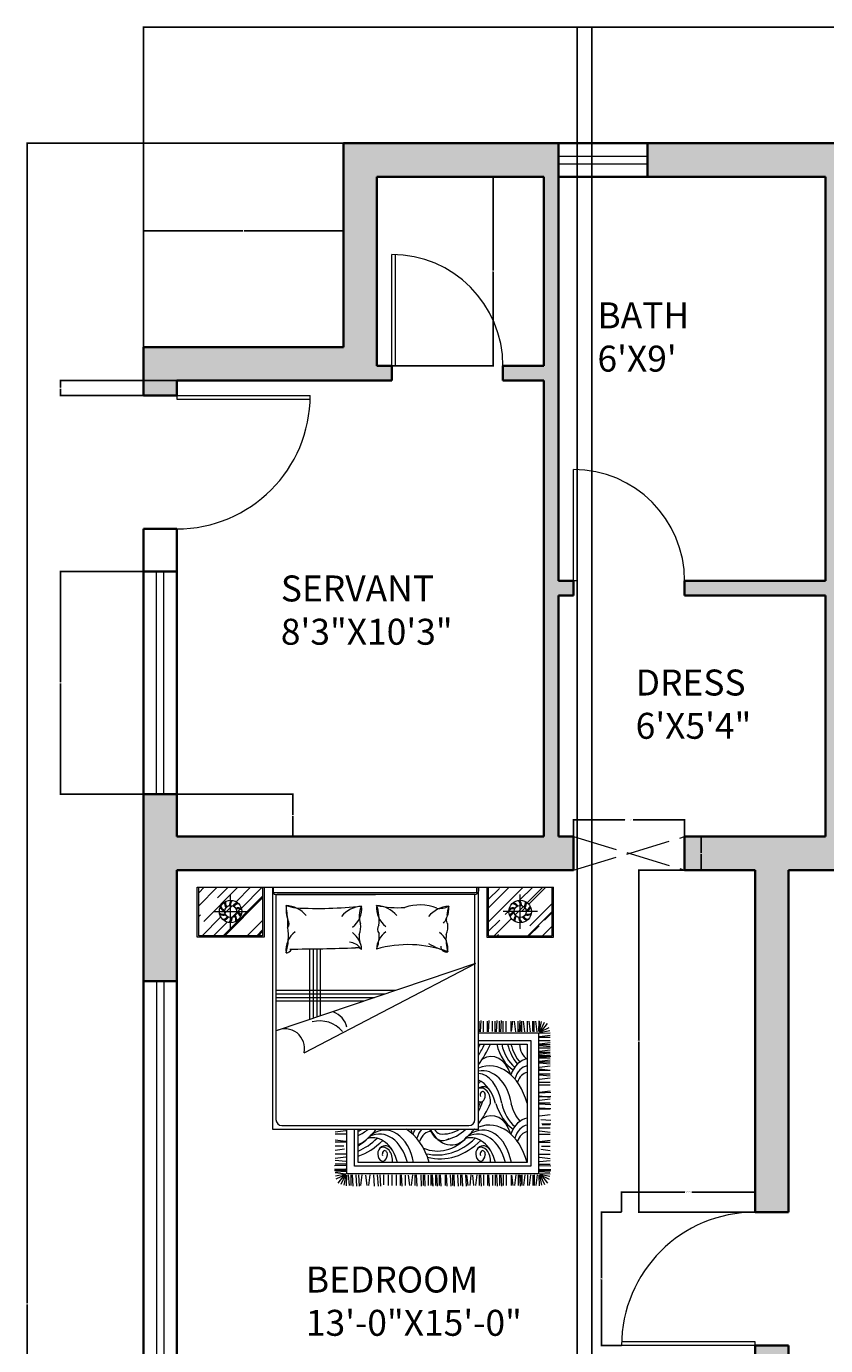
# Model space of a CAD drawing. Units: inches. Extents: x 1919 to 2461, y 2470 to 3159.
# Tile 4 of 6: x 1919 to 2134, y 2803 to 3159. Entities that reach past the tile are written whole.
import ezdxf

# ---------------------------------------------------------------- set-up
doc = ezdxf.new("R2010")
doc.units = ezdxf.units.IN
doc.linetypes.add('ACAD_ISO02W100', pattern=[15, 12, -3])
for name, color, linetype, lineweight in [('A-ANNO-DIMS', 2, 'Continuous', 18), ('A-AREA-IDEN', 7, 'Continuous', 18), ('A-DOOR', 3, 'Continuous', 18), ('A-FURN', 8, 'Continuous', 18), ('A-GLAZ', 4, 'Continuous', 18), ('A-WALL', 7, 'Continuous', 35), ('A-WALL-OVHD', 7, 'ACAD_ISO02W100', 13), ('A-WALL-PATT', 252, 'Continuous', 13)]:
    doc.layers.add(name, color=color, linetype=linetype, lineweight=lineweight)
doc.styles.get("Standard").update_dxf_attribs({"font": 'arial.ttf'})
doc.dimstyles.get("Standard").update_dxf_attribs({"dimtxt": 0.18, "dimasz": 0.18, "dimexe": 0.18, "dimexo": 0.0625, "dimgap": 0.09, "dimtad": 0, "dimtih": 1, "dimtoh": 1, "dimdec": 4, "dimzin": 0, "dimdsep": 46, "dimtxsty": 'Standard', "dimcen": 0.09, "dimadec": 0, "dimazin": 0, "dimtfac": 1, "dimtdec": 4, "dimtofl": 0, "dimtmove": 0, "dimatfit": 3, "dimfxl": 1, "dimtolj": 1, "dimtzin": 0, "dimarcsym": 0})

# ---------------------------------------------------------------- blocks, each defined once
blk = doc.blocks.new('A$C64B41DC1')
for p, q in [((0, 2.508), (2.99, 2.508)), ((0, 2.088), (0, 2.508)), ((0.012, 2.462), (0.058, 2.508)), ((0.012, 2.352), (0.168, 2.508)), ((0.012, 2.1), (0.012, 2.508)), ((0.054, 2.221), (0.341, 2.508)), ((0.169, 2.418), (0.259, 2.508)), ((0.28, 2.16), (0.28, 2.448)), ((0.327, 2.386), (0.448, 2.508)), ((0.37, 2.333), (0.545, 2.508)), ((0.548, 2.508), (0.548, 2.1)), ((0.56, 2.508), (0.56, 2.088)), ((0.63, 2.508), (0.63, 0.478)), ((0.64, 2.461), (0.64, 2.508)), ((0.64, 2.508), (2.344, 2.508)), ((2.344, 2.461), (0.64, 2.461)), ((0.66, 2.446), (1.495, 2.446)), ((0.66, 2.446), (0.66, 0.558)), ((1.495, 2.446), (0.67, 2.446)), ((2.33, 2.446), (1.495, 2.446)), ((2.33, 0.558), (2.33, 2.446)), ((2.344, 2.508), (2.36, 2.508)), ((2.344, 2.508), (2.344, 2.461)), ((2.36, 2.508), (2.36, 2.476)), ((2.36, 0.478), (2.36, 2.508)), ((2.43, 2.508), (2.43, 2.088)), ((2.442, 2.508), (2.442, 2.1)), ((2.442, 2.333), (2.617, 2.508)), ((2.442, 2.214), (2.736, 2.508)), ((2.442, 2.404), (2.535, 2.497)), ((2.705, 2.398), (2.815, 2.508)), ((2.71, 2.16), (2.71, 2.448)), ((2.769, 2.377), (2.9, 2.508)), ((2.782, 2.365), (2.925, 2.508)), ((2.978, 2.1), (2.978, 2.508)), ((2.99, 2.088), (2.99, 2.508)), ((0.216, 2.1), (0.548, 2.432)), ((0.23, 2.1), (0.548, 2.418)), ((0.231, 2.291), (0.294, 2.353)), ((2.667, 2.276), (2.738, 2.346)), ((2.725, 2.308), (2.751, 2.334)), ((2.791, 2.185), (2.978, 2.371)), ((0.012, 2.261), (0.027, 2.276)), ((0.04, 2.1), (0.198, 2.258)), ((0.136, 2.304), (0.425, 2.304)), ((0.137, 2.1), (0.251, 2.214)), ((0.291, 2.254), (0.33, 2.294)), ((0.341, 2.304), (0.36, 2.324)), ((0.419, 2.1), (0.548, 2.229)), ((2.442, 2.135), (2.538, 2.231)), ((2.492, 2.1), (2.637, 2.245)), ((2.854, 2.304), (2.566, 2.304)), ((2.585, 2.278), (2.616, 2.309)), ((2.616, 2.309), (2.631, 2.324)), ((2.775, 2.1), (2.978, 2.304)), ((2.914, 2.231), (2.978, 2.295)), ((0.499, 2.1), (0.548, 2.149)), ((0.513, 2.1), (0.548, 2.135)), ((2.517, 2.1), (2.527, 2.11)), ((2.783, 2.1), (2.868, 2.185)), ((2.896, 2.1), (2.978, 2.182)), ((0.56, 2.088), (0, 2.088)), ((0.548, 2.1), (0.012, 2.1)), ((2.43, 2.088), (2.99, 2.088)), ((2.442, 2.1), (2.978, 2.1)), ((0.942, 1.99), (0.942, 1.397)), ((0.972, 1.991), (0.972, 1.408)), ((1.002, 1.991), (1.002, 1.418)), ((1.032, 1.992), (1.032, 1.428)), ((2.335, 1.868), (0.661, 1.303)), ((0.896, 1.119), (2.335, 1.868)), ((1.664, 1.641), (0.66, 1.641)), ((1.575, 1.611), (0.66, 1.611)), ((2.366, 1.295), (2.366, 1.384)), ((2.377, 1.295), (2.382, 1.389)), ((2.403, 1.295), (2.403, 1.384)), ((2.435, 1.295), (2.435, 1.384)), ((2.445, 1.295), (2.45, 1.389)), ((2.477, 1.296), (2.477, 1.384)), ((2.5, 1.295), (2.5, 1.384)), ((2.51, 1.295), (2.516, 1.389)), ((2.537, 1.295), (2.537, 1.384)), ((2.547, 1.295), (2.552, 1.389)), ((2.568, 1.295), (2.568, 1.384)), ((2.592, 1.295), (2.592, 1.384)), ((2.635, 1.296), (2.635, 1.384)), ((2.636, 1.296), (2.647, 1.384)), ((2.673, 1.295), (2.662, 1.384)), ((2.694, 1.295), (2.694, 1.384)), ((2.704, 1.295), (2.71, 1.389)), ((2.713, 1.296), (2.723, 1.384)), ((2.725, 1.295), (2.725, 1.384)), ((2.749, 1.295), (2.739, 1.384)), ((2.772, 1.295), (2.772, 1.384)), ((2.796, 1.295), (2.785, 1.384)), ((2.815, 1.296), (2.815, 1.384)), ((2.815, 1.296), (2.815, 1.384)), ((2.828, 1.295), (2.828, 1.384)), ((2.828, 1.295), (2.828, 1.384)), ((2.852, 1.295), (2.842, 1.384)), ((2.852, 1.295), (2.842, 1.384)), ((2.865, 1.297), (2.869, 1.386)), ((2.871, 1.296), (2.871, 1.384)), ((2.871, 1.296), (2.888, 1.382)), ((2.871, 1.293), (2.954, 1.332)), ((2.877, 1.296), (2.913, 1.376)), ((2.889, 1.301), (2.939, 1.364)), ((2.36, 1.287), (2.864, 1.287)), ((2.36, 1.223), (2.8, 1.223)), ((2.8, 1.223), (2.8, 0.166)), ((2.864, 1.287), (2.864, 0.102)), ((2.872, 1.288), (2.959, 1.306)), ((2.872, 1.256), (2.96, 1.267)), ((2.872, 1.249), (2.96, 1.249)), ((2.872, 1.221), (2.96, 1.221)), ((2.874, 1.282), (2.96, 1.287)), ((2.36, 1.191), (2.768, 1.191)), ((2.768, 1.191), (2.768, 0.198)), ((2.872, 1.195), (2.96, 1.205)), ((2.872, 1.187), (2.96, 1.187)), ((2.872, 1.181), (2.96, 1.171)), ((2.872, 1.159), (2.96, 1.159)), ((2.872, 1.133), (2.96, 1.143)), ((2.872, 1.125), (2.96, 1.125)), ((2.872, 1.119), (2.96, 1.109)), ((2.872, 1.104), (2.96, 1.093)), ((2.872, 1.097), (2.96, 1.097)), ((2.872, 1.086), (2.966, 1.091)), ((2.872, 1.086), (2.96, 1.075)), ((2.872, 1.076), (2.96, 1.076)), ((2.872, 1.049), (2.96, 1.06)), ((2.872, 1.042), (2.96, 1.042)), ((2.872, 1.035), (2.96, 1.025)), ((2.872, 0.999), (2.96, 1.009)), ((2.872, 0.985), (2.96, 0.974)), ((2.872, 0.973), (2.96, 0.973)), ((2.872, 0.941), (2.96, 0.941)), ((2.872, 0.935), (2.96, 0.924)), ((2.872, 0.898), (2.96, 0.908)), ((2.872, 0.873), (2.96, 0.873)), ((2.872, 0.85), (2.96, 0.85)), ((2.872, 0.789), (2.96, 0.799)), ((2.872, 0.782), (2.966, 0.787)), ((2.872, 0.757), (2.96, 0.747)), ((2.872, 0.75), (2.966, 0.756)), ((2.872, 0.72), (2.96, 0.731)), ((2.872, 0.699), (2.96, 0.699)), ((2.872, 0.689), (2.966, 0.684)), ((2.872, 0.658), (2.966, 0.652)), ((2.872, 0.647), (2.96, 0.647)), ((2.872, 0.59), (2.96, 0.601)), ((2.882, 0.558), (2.966, 0.554)), ((0.63, 0.478), (2.36, 0.478)), ((0.71, 0.508), (2.28, 0.508)), ((1.246, 0.463), (1.158, 0.452)), ((1.254, 0.102), (1.254, 0.478)), ((1.318, 0.166), (1.318, 0.478)), ((1.35, 0.198), (1.35, 0.478)), ((2.872, 0.488), (2.96, 0.488)), ((2.872, 0.463), (2.96, 0.452)), ((2.891, 0.526), (2.966, 0.522)), ((2.893, 0.517), (2.96, 0.517)), ((1.246, 0.437), (1.158, 0.437)), ((1.246, 0.375), (1.158, 0.385)), ((1.246, 0.368), (1.158, 0.368)), ((1.229, 0.336), (1.158, 0.336)), ((2.872, 0.437), (2.96, 0.437)), ((2.872, 0.375), (2.96, 0.385)), ((2.872, 0.368), (2.96, 0.368)), ((2.89, 0.336), (2.96, 0.336)), ((1.235, 0.309), (1.158, 0.3)), ((1.246, 0.268), (1.158, 0.268)), ((1.246, 0.242), (1.158, 0.232)), ((2.872, 0.268), (2.96, 0.268)), ((2.872, 0.242), (2.96, 0.232)), ((2.883, 0.309), (2.96, 0.3)), ((1.246, 0.174), (1.152, 0.169)), ((1.246, 0.143), (1.152, 0.138)), ((1.246, 0.133), (1.152, 0.128)), ((1.246, 0.206), (1.158, 0.216)), ((1.246, 0.185), (1.158, 0.185)), ((1.246, 0.132), (1.158, 0.132)), ((1.246, 0.132), (1.158, 0.132)), ((1.246, 0.123), (1.159, 0.117)), ((2.8, 0.166), (1.318, 0.166)), ((2.768, 0.198), (1.35, 0.198)), ((2.872, 0.206), (2.96, 0.216)), ((2.872, 0.185), (2.96, 0.185)), ((2.872, 0.174), (2.966, 0.169)), ((2.872, 0.143), (2.966, 0.138)), ((2.872, 0.133), (2.966, 0.128)), ((2.872, 0.132), (2.96, 0.132)), ((2.872, 0.123), (2.959, 0.117)), ((1.246, 0.1), (1.158, 0.11)), ((1.246, 0.101), (1.159, 0.083)), ((1.247, 0.096), (1.164, 0.058)), ((1.229, 0.088), (1.179, 0.026)), ((1.242, 0.093), (1.205, 0.013)), ((1.247, 0.093), (1.231, 0.007)), ((1.253, 0.092), (1.249, 0.003)), ((2.864, 0.102), (1.254, 0.102)), ((1.266, 0.094), (1.276, 0.005)), ((1.29, 0.094), (1.29, 0.005)), ((1.3, 0.094), (1.305, 0)), ((1.331, 0.094), (1.337, 0)), ((1.352, 0.094), (1.358, 0)), ((1.38, 0.094), (1.37, 0.005)), ((1.412, 0.093), (1.422, 0.005)), ((1.449, 0.094), (1.438, 0.005)), ((1.48, 0.094), (1.485, 0)), ((1.511, 0.094), (1.517, 0)), ((1.532, 0.094), (1.538, 0)), ((1.564, 0.094), (1.564, 0.01)), ((1.602, 0.094), (1.602, 0.005)), ((1.634, 0.094), (1.634, 0.005)), ((1.67, 0.094), (1.67, 0.005)), ((1.702, 0.094), (1.702, 0.005)), ((1.712, 0.094), (1.717, 0)), ((1.745, 0.093), (1.745, 0.005)), ((1.77, 0.093), (1.78, 0.005)), ((1.806, 0.094), (1.796, 0.005)), ((1.827, 0.094), (1.827, 0.005)), ((1.838, 0.094), (1.843, 0)), ((1.875, 0.094), (1.88, 0)), ((1.896, 0.094), (1.896, 0.005)), ((1.906, 0.094), (1.911, 0)), ((1.938, 0.093), (1.938, 0.005)), ((1.961, 0.094), (1.961, 0.005)), ((1.964, 0.093), (1.974, 0.005)), ((1.971, 0.094), (1.977, 0)), ((1.998, 0.094), (1.998, 0.005)), ((2.008, 0.094), (2.013, 0)), ((2.029, 0.094), (2.029, 0.005)), ((2.039, 0.094), (2.045, 0)), ((2.08, 0.094), (2.08, 0.005)), ((2.09, 0.094), (2.095, 0)), ((2.122, 0.094), (2.127, 0)), ((2.141, 0.094), (2.141, 0.005)), ((2.152, 0.094), (2.157, 0)), ((2.183, 0.094), (2.188, 0)), ((2.209, 0.094), (2.209, 0.005)), ((2.22, 0.094), (2.225, 0)), ((2.251, 0.094), (2.256, 0)), ((2.26, 0.093), (2.271, 0.005)), ((2.297, 0.094), (2.286, 0.005)), ((2.309, 0.093), (2.319, 0.005)), ((2.346, 0.094), (2.335, 0.005)), ((2.366, 0.094), (2.366, 0.005)), ((2.377, 0.094), (2.382, 0)), ((2.403, 0.094), (2.403, 0.005)), ((2.435, 0.094), (2.435, 0.005)), ((2.445, 0.094), (2.45, 0)), ((2.477, 0.093), (2.477, 0.005)), ((2.5, 0.094), (2.5, 0.005)), ((2.51, 0.094), (2.516, 0)), ((2.537, 0.094), (2.537, 0.005)), ((2.547, 0.094), (2.552, 0)), ((2.568, 0.094), (2.568, 0.005)), ((2.592, 0.094), (2.592, 0.005)), ((2.635, 0.093), (2.635, 0.005)), ((2.636, 0.093), (2.647, 0.005)), ((2.673, 0.094), (2.662, 0.005)), ((2.694, 0.094), (2.694, 0.005)), ((2.704, 0.094), (2.71, 0)), ((2.713, 0.093), (2.723, 0.005)), ((2.725, 0.094), (2.725, 0.005)), ((2.749, 0.094), (2.739, 0.005)), ((2.772, 0.094), (2.772, 0.005)), ((2.796, 0.094), (2.785, 0.005)), ((2.815, 0.093), (2.815, 0.005)), ((2.828, 0.094), (2.828, 0.005)), ((2.852, 0.094), (2.842, 0.005)), ((2.865, 0.092), (2.869, 0.003)), ((2.871, 0.096), (2.954, 0.058)), ((2.871, 0.093), (2.888, 0.007)), ((2.872, 0.101), (2.959, 0.083)), ((2.874, 0.107), (2.96, 0.102)), ((2.877, 0.093), (2.913, 0.013)), ((2.889, 0.088), (2.939, 0.026))]:
    blk.add_line(p, q)
at = {"ltscale": 10}
for p, q in [((1.486, 1.581), (0.66, 1.581)), ((1.397, 1.551), (0.66, 1.551))]:
    blk.add_line(p, q, dxfattribs=at)
for centre, radius in [((0.28, 2.304), 0.0942), ((0.28, 2.304), 0.051), ((2.71, 2.304), 0.0942), ((2.71, 2.304), 0.051)]:
    blk.add_circle(centre, radius)
for centre, radius, start, end in [((0.66, 2.476), 0.03, 180, 270), ((2.33, 2.476), 0.03, 270, 0), ((0.246, 2.366), 0.0605, 208.17, 254.4897), ((0.242, 2.361), 0.0462, 196.3002, 256.538), ((0.289, 2.374), 0.0605, 172.17, 218.4897), ((0.283, 2.373), 0.0462, 160.3002, 220.538), ((0.329, 2.356), 0.0605, 136.17, 182.4897), ((0.323, 2.358), 0.0462, 124.3002, 184.538), ((0.35, 2.318), 0.0605, 100.17, 146.4897), ((0.347, 2.323), 0.0462, 88.3002, 148.538), ((0.345, 2.274), 0.0605, 64.17, 110.4897), ((0.345, 2.28), 0.0462, 52.3002, 112.538), ((1.053, 2.33), 0.308, 175.3048, 198.6942), ((-0.87, 2.094), 1.636, 4.8098, 9.1892), ((0.858, 2.628), 0.295, 247.5179, 264.267), ((0.728, 2.111), 0.245, 40.4189, 85.9871), ((1.016, 5.71), 3.38, 266.8134, 276.1602), ((1.396, 2.104), 0.245, 94.0129, 139.5811), ((1.186, 2.329), 0.194, 306.5711, 5.89), ((1.535, 2.265), 0.177, 151.7736, 201.6983), ((1.699, 2.335), 0.194, 174.11, 233.4289), ((1.148, 2.231), 0.378, 353.4947, 19.1867), ((1.687, 3.192), 0.856, 257.7438, 273.6284), ((1.488, 2.111), 0.245, 40.4189, 85.9871), ((1.867, 1.971), 0.388, 68.2026, 108.9817), ((2.127, 2.104), 0.245, 94.0129, 139.5811), ((2.034, 2.486), 0.156, 261.5958, 298.9092), ((1.916, 2.329), 0.194, 333.7371, 5.89), ((2.606, 2.203), 0.517, 163.6046, 172.3273), ((2.645, 2.28), 0.0462, 67.462, 127.6998), ((2.645, 2.274), 0.0605, 69.5103, 115.83), ((2.643, 2.323), 0.0462, 31.462, 91.6998), ((2.64, 2.318), 0.0605, 33.5103, 79.83), ((2.667, 2.358), 0.0462, 355.462, 55.6998), ((2.662, 2.356), 0.0605, 357.5103, 43.83), ((2.707, 2.373), 0.0462, 319.462, 19.6998), ((2.702, 2.374), 0.0605, 321.5103, 7.83), ((2.749, 2.361), 0.0462, 283.462, 343.6998), ((2.745, 2.366), 0.0605, 285.5103, 331.83), ((0.215, 2.328), 0.0462, 232.3002, 292.538), ((0.216, 2.334), 0.0605, 244.17, 290.4897), ((0.214, 2.285), 0.0462, 268.3002, 328.538), ((0.211, 2.29), 0.0605, 280.17, 326.4897), ((0.238, 2.249), 0.0462, 304.3002, 4.538), ((0.232, 2.252), 0.0605, 316.17, 2.4897), ((0.278, 2.235), 0.0462, 340.3002, 40.538), ((0.272, 2.233), 0.0605, 352.17, 38.4897), ((0.319, 2.246), 0.0462, 16.3002, 76.538), ((0.315, 2.242), 0.0605, 28.17, 74.4897), ((0.727, 2.201), 0.0446, 314.4736, 42.1713), ((-1.601, 2.277), 2.362, 357.3905, 358.8876), ((1.916, 2.329), 0.194, 320.9404, 333.7371), ((2.135, 2.231), 0.0459, 165.3506, 223.2684), ((2.675, 2.242), 0.0605, 105.5103, 151.83), ((2.671, 2.246), 0.0462, 103.462, 163.6998), ((2.718, 2.233), 0.0605, 141.5103, 187.83), ((2.712, 2.235), 0.0462, 139.462, 199.6998), ((2.758, 2.252), 0.0605, 177.5103, 223.83), ((2.753, 2.249), 0.0462, 175.462, 235.6998), ((2.78, 2.29), 0.0605, 213.5103, 259.83), ((2.777, 2.285), 0.0462, 211.462, 271.6998), ((2.774, 2.334), 0.0605, 249.5103, 295.83), ((2.775, 2.328), 0.0462, 247.462, 307.6998), ((0.938, 1.978), 0.194, 126.5711, 185.89), ((0.269, 2.094), 0.496, 344.0243, 8.7071), ((1.186, 1.971), 0.194, 4.3181, 53.4289), ((1.541, 2.097), 0.183, 175.2233, 196.23), ((1.204, 2.178), 0.168, 337.017, 7.5368), ((1.706, 1.971), 0.204, 127.1197, 175.09), ((1.567, 2.155), 0.0547, 142.0833, 220.902), ((1.196, 2.098), 0.33, 343.7954, 3.5554), ((1.939, 1.991), 0.165, 351.2621, 55.7572), ((2.462, 2.072), 0.375, 173.8296, 196.4356), ((1.935, 2.178), 0.168, 337.017, 7.5368), ((0.725, 18.844), 16.855, 270.174, 272.0521), ((1.269, 1.925), 0.122, 33.628, 86.4744), ((1.34, 1.94), 0.0603, 49.0991, 101.3702), ((1.768, 1.063), 0.963, 69.6507, 105.9631), ((2.275, 2.579), 0.637, 238.3499, 254.3137), ((2.091, 2.012), 0.0478, 179.7727, 283.8018), ((0.742, 2.015), 0.057, 273.4709, 328.5412), ((0.728, 2.202), 0.245, 274.0129, 278.3417), ((1.075, 1.287), 0.187, 14.1863, 69.1212), ((1.027, 1.133), 0.253, 40.629, 104.3712), ((0.735, 1.155), 0.165, 347.3109, 116.4454), ((0.71, 0.558), 0.05, 180, 270), ((2.28, 0.558), 0.05, 270, 0)]:
    blk.add_arc(centre, radius, start, end)
for centre, major_axis, ratio, start_param, end_param in [((1.994, 1.626), (0, -0.753), 0.68, 0.797284, 0.954936), ((2.064, 1.466), (0, -0.532), 0.68, 7.239912, 7.311536), ((1.905, 1.74), (0, -0.984), 0.68, 0.74745, 0.979724), ((2.467, 0.822), (0, -0.266), 0.68, 2.006169, 3.565187), ((2.746, 1.308), (0, 0.361), 0.68, 1.900046, 2.742661), ((2.787, 1.308), (0, 0.361), 0.68, 1.900046, 2.614747), ((2.837, 1.308), (0, 0.361), 0.68, 1.900046, 2.479658), ((2.861, 1.321), (0, 0.361), 0.68, 1.938265, 2.479658), ((2.806, 1.208), (0, -0.152), 0.68, 4.821745, 5.895886), ((2.451, 0.507), (0, 0.502), 0.68, 5.095327, 6.553458), ((2.786, 0.807), (0, -0.261), 0.68, 3.244645, 4.205018), ((2.778, 0.829), (0, -0.18), 0.68, 3.227058, 4.318474), ((2.396, 0.603), (0, 0.364), 0.68, -1.3172, 0.145284), ((2.351, 0.564), (0.007, 0.382), 0.56205, -1.21172, -0.009991), ((2.296, 0.577), (0, -0.326), 0.68, 1.938944, 2.850232), ((2.782, 0.797), (0, -0.159), 0.68, 3.272942, 4.229533), ((2.04, 1.601), (0, -0.876), 0.68, 6.849801, 6.887077), ((2.4, 0.713), (0, -0.121), 0.68, 2.284368, 3.652258), ((2.383, 0.708), (0, 0.115), 0.68, 4.593909, 6.585576), ((2.396, 0.763), (0, -0.0317), 0.68, 1.462497, 5.046281), ((2.377, 0.765), (0, -0.0593), 0.68, 5.841311, 7.755362), ((1.994, 1.13), (-0.068, 0.744), 0.610498, 3.917146, 4.063997), ((2.064, 0.969), (0, -0.532), 0.68, 7.239912, 7.336618), ((1.905, 1.243), (0, -0.984), 0.68, 0.74745, 0.979724), ((2.746, 0.811), (-0.06, 0.373), 0.695517, 1.775813, 2.548612), ((2.787, 0.811), (0, 0.361), 0.68, 1.900046, 2.614747), ((2.861, 0.824), (0, 0.361), 0.68, 1.938265, 2.479658), ((2.451, 0.01), (0, 0.502), 0.68, 5.095327, 6.553458), ((2.467, 0.325), (0, -0.266), 0.68, 2.006169, 3.565187), ((2.786, 0.31), (0, -0.261), 0.68, 3.244645, 4.205018), ((1.242, 0.969), (0, -0.532), 0.68, 6.586764, 6.677612), ((1.171, 1.13), (-0.116, 0.724), 0.59432, 3.291697, 3.50733), ((1.083, 1.243), (0, -0.984), 0.68, 0.565948, 0.680366), ((1.528, 0.067), (0, -0.37), 0.68, 1.930561, 3.464283), ((1.574, 0.106), (0, 0.364), 0.68, -1.3172, 0.476403), ((1.629, 0.01), (0, 0.502), 0.68, 6.655152, 6.661293), ((1.629, 0.01), (0, 0.502), 0.68, 5.095327, 5.911219), ((1.644, 0.325), (0, -0.266), 0.68, 2.006169, 2.182797), ((1.964, 0.31), (0, -0.261), 0.68, 4.015924, 4.205018), ((1.956, 0.332), (0, -0.18), 0.68, 3.770744, 4.318474), ((1.96, 0.3), (0, -0.159), 0.68, 3.14258, 4.229533), ((2.061, 0.562), (0, -0.18), 0.68, 5.194792, 5.929328), ((2.061, 0.562), (0, -0.18), 0.68, 5.194792, 6.723255), ((2.131, 0.66), (0, -0.315), 0.68, 5.328638, 6.949396), ((2.055, 0.566), (0, -0.13), 0.68, 5.450951, 6.054641), ((2.064, 0.969), (0, -0.532), 0.68, 6.20013, 6.677612), ((1.994, 1.13), (-0.068, 0.744), 0.610498, 3.199135, 3.592282), ((1.905, 1.243), (0, -0.984), 0.68, 0.565948, 0.680366), ((2.351, 0.067), (0, -0.37), 0.68, 1.930561, 3.464283), ((2.396, 0.106), (0, 0.364), 0.68, -1.3172, 0.476403), ((2.451, 0.01), (0, 0.502), 0.68, 6.655152, 6.661293), ((2.778, 0.332), (0, -0.18), 0.68, 3.227058, 4.318474), ((2.782, 0.3), (0, -0.159), 0.68, 3.272942, 4.229533), ((1.193, 0.918), (0, -0.624), 0.68, 0.378672, 0.625379), ((1.309, 0.66), (0, -0.315), 0.68, 6.475719, 6.949396), ((1.191, 1.107), (0, 0.846), 0.68, 3.421828, 3.728616), ((1.218, 1.105), (0, -0.876), 0.68, 6.507006, 6.887077), ((1.474, 0.08), (0, -0.326), 0.68, 1.938944, 3.339184), ((1.578, 0.217), (0, -0.121), 0.68, 2.284368, 3.726131), ((1.561, 0.211), (0, 0.115), 0.68, 4.593909, 6.647252), ((2.016, 0.918), (0, -0.624), 0.68, -0.280078, 0.625379), ((2.013, 1.107), (0, 0.846), 0.68, 2.978727, 3.728616), ((2.04, 1.105), (0, -0.876), 0.68, 6.099302, 6.887077), ((2.296, 0.08), (0, -0.326), 0.68, 1.938944, 3.339184), ((2.4, 0.217), (0, -0.121), 0.68, 2.284368, 3.726131), ((2.383, 0.211), (0, 0.115), 0.68, 4.593909, 6.647252), ((1.555, 0.269), (0, -0.0593), 0.68, 3.732151, 7.755362), ((1.574, 0.266), (0, -0.0317), 0.68, 1.462497, 5.046281), ((2.377, 0.269), (0, -0.0593), 0.68, 3.732151, 7.755362), ((2.396, 0.266), (0, -0.0317), 0.68, 1.462497, 5.046281)]:
    blk.add_ellipse(centre, major_axis=major_axis, ratio=ratio, start_param=start_param, end_param=end_param)
blk = doc.blocks.new('DOOR-SGL-30IN')
for p, q in [((0, 0), (0, 30)), ((1, 0), (1, 29.98)), ((1, 0), (0, 0))]:
    blk.add_line(p, q)
blk.add_arc((0, 0), 30, 0, 90)
blk = doc.blocks.new('DOOR-SGL-36IN')
for p, q in [((0, 0), (-36, 0)), ((0, 1), (-35.99, 1)), ((0, 0), (0, 1))]:
    blk.add_line(p, q)
blk.add_arc((0, 0), 36, 90, 180)
blk = doc.blocks.new('WIN-GLAZ-120IN')
for p, q in [((120, 0), (0, 0)), ((120, -2), (0, -2))]:
    blk.add_line(p, q)
blk = doc.blocks.new('WIN-GLAZ-24IN')
for p, q in [((-2, 24), (-2, 0)), ((0, 24), (0, 0))]:
    blk.add_line(p, q)
blk = doc.blocks.new('OPENING-OVHD-30IN')
for p, q in [((0, 0), (9, 30)), ((9, 0), (0, 30))]:
    blk.add_line(p, q)
blk = doc.blocks.new('*D13')
at = {"layer": 'A-ANNO-DIMS', "color": 0, "lineweight": -2, "transparency": 16777216}
for p, q in [((2079.32, 2839.46), (2079.32, 2844.98)), ((2079.5, 2844.8), (2096.38, 2844.8)), ((2115.14, 2844.8), (2098.25, 2844.8)), ((2115.32, 2839.46), (2115.32, 2844.98))]:
    blk.add_line(p, q, dxfattribs=at)
at = {"layer": 'A-ANNO-DIMS', "color": 0, "transparency": 16777216}
for points in [[(2079.5, 2844.83), (2079.5, 2844.77), (2079.32, 2844.8)], [(2115.14, 2844.83), (2115.14, 2844.77), (2115.32, 2844.8)]]:
    blk.add_solid(points, dxfattribs=at)
at = {"layer": 'Defpoints', "color": 0, "transparency": 16777216}
for p in [(2115.32, 2844.8), (2079.32, 2839.4), (2115.32, 2839.4)]:
    blk.add_point(p, dxfattribs=at)
at = {"layer": 'A-ANNO-DIMS', "color": 0, "transparency": 16777216, "insert": (2097.32, 2844.8), "char_height": 0.18, "attachment_point": 5}
blk.add_mtext('\\A1;DOOR 36 TYP.', dxfattribs=at)
blk = doc.blocks.new('*D14')
at = {"layer": 'A-ANNO-DIMS', "color": 0, "lineweight": -2, "transparency": 16777216}
for p, q in [((2079.25, 2839.4), (2073.74, 2839.4)), ((2073.92, 2839.22), (2073.92, 2821.58)), ((2073.92, 2803.58), (2073.92, 2821.22)), ((2079.25, 2803.4), (2073.74, 2803.4))]:
    blk.add_line(p, q, dxfattribs=at)
at = {"layer": 'A-ANNO-DIMS', "color": 0, "transparency": 16777216}
for points in [[(2073.89, 2839.22), (2073.95, 2839.22), (2073.92, 2839.4)], [(2073.89, 2803.58), (2073.95, 2803.58), (2073.92, 2803.4)]]:
    blk.add_solid(points, dxfattribs=at)
at = {"layer": 'Defpoints', "color": 0, "transparency": 16777216}
for p in [(2073.92, 2839.4), (2079.32, 2839.4), (2079.32, 2803.4)]:
    blk.add_point(p, dxfattribs=at)
at = {"layer": 'A-ANNO-DIMS', "color": 0, "transparency": 16777216, "insert": (2073.92, 2821.4), "char_height": 0.18, "attachment_point": 5}
blk.add_mtext('\\A1;36 TYP.', dxfattribs=at)
blk = doc.blocks.new('*D21')
at = {"layer": 'A-ANNO-DIMS', "color": 0, "lineweight": -2, "transparency": 16777216}
for p, q in [((2066.32, 2940.73), (2066.32, 2945.35)), ((2066.5, 2945.17), (2080.17, 2945.17)), ((2096.14, 2945.17), (2082.46, 2945.17)), ((2096.32, 2940.73), (2096.32, 2945.35))]:
    blk.add_line(p, q, dxfattribs=at)
at = {"layer": 'A-ANNO-DIMS', "color": 0, "transparency": 16777216}
for points in [[(2066.5, 2945.2), (2066.5, 2945.14), (2066.32, 2945.17)], [(2096.14, 2945.2), (2096.14, 2945.14), (2096.32, 2945.17)]]:
    blk.add_solid(points, dxfattribs=at)
at = {"layer": 'Defpoints', "color": 0, "transparency": 16777216}
for p in [(2096.32, 2945.17), (2066.32, 2940.67), (2096.32, 2940.67)]:
    blk.add_point(p, dxfattribs=at)
at = {"layer": 'A-ANNO-DIMS', "color": 0, "transparency": 16777216, "insert": (2081.32, 2945.17), "char_height": 0.18, "attachment_point": 5}
blk.add_mtext('\\A1;OPENING 30 TYP.', dxfattribs=at)
blk = doc.blocks.new('*D22')
at = {"layer": 'A-ANNO-DIMS', "color": 0, "lineweight": -2, "transparency": 16777216}
for p, q in [((2096.38, 2940.67), (2101, 2940.67)), ((2100.82, 2940.49), (2100.82, 2936.35)), ((2100.82, 2931.85), (2100.82, 2935.99)), ((2096.38, 2931.67), (2101, 2931.67))]:
    blk.add_line(p, q, dxfattribs=at)
at = {"layer": 'A-ANNO-DIMS', "color": 0, "transparency": 16777216}
for points in [[(2100.79, 2940.49), (2100.85, 2940.49), (2100.82, 2940.67)], [(2100.79, 2931.85), (2100.85, 2931.85), (2100.82, 2931.67)]]:
    blk.add_solid(points, dxfattribs=at)
at = {"layer": 'Defpoints', "color": 0, "transparency": 16777216}
for p in [(2096.32, 2940.67), (2096.32, 2931.67), (2100.82, 2931.67)]:
    blk.add_point(p, dxfattribs=at)
at = {"layer": 'A-ANNO-DIMS', "color": 0, "transparency": 16777216, "insert": (2100.82, 2936.17), "char_height": 0.18, "attachment_point": 5}
blk.add_mtext('\\A1;9 TYP.', dxfattribs=at)
blk = doc.blocks.new('*D23')
at = {"layer": 'A-ANNO-DIMS', "color": 0, "lineweight": -2, "transparency": 16777216}
for p, q in [((1950.32, 3072.73), (1950.32, 3159.21)), ((1950.5, 3159.03), (2189.52, 3159.03)), ((2429.14, 3159.03), (2190.11, 3159.03)), ((2429.32, 3127.73), (2429.32, 3159.21))]:
    blk.add_line(p, q, dxfattribs=at)
at = {"layer": 'A-ANNO-DIMS', "color": 0, "transparency": 16777216}
for points in [[(1950.5, 3159.06), (1950.5, 3159), (1950.32, 3159.03)], [(2429.14, 3159.06), (2429.14, 3159), (2429.32, 3159.03)]]:
    blk.add_solid(points, dxfattribs=at)
at = {"layer": 'Defpoints', "color": 0, "transparency": 16777216}
for p in [(2429.32, 3159.03), (2429.32, 3127.67), (1950.32, 3072.67)]:
    blk.add_point(p, dxfattribs=at)
at = {"layer": 'A-ANNO-DIMS', "color": 0, "transparency": 16777216, "insert": (2189.82, 3159.03), "char_height": 0.18, "attachment_point": 5}
blk.add_mtext('\\A1;479', dxfattribs=at)
blk = doc.blocks.new('*D24')
at = {"layer": 'A-ANNO-DIMS', "color": 0, "lineweight": -2, "transparency": 16777216}
for p, q in [((2004.25, 3127.67), (1918.78, 3127.67)), ((1918.96, 3127.49), (1918.96, 2814.85)), ((1918.96, 2501.85), (1918.96, 2814.49)), ((1950.25, 2501.67), (1918.78, 2501.67))]:
    blk.add_line(p, q, dxfattribs=at)
at = {"layer": 'A-ANNO-DIMS', "color": 0, "transparency": 16777216}
for points in [[(1918.93, 3127.49), (1918.99, 3127.49), (1918.96, 3127.67)], [(1918.93, 2501.85), (1918.99, 2501.85), (1918.96, 2501.67)]]:
    blk.add_solid(points, dxfattribs=at)
at = {"layer": 'Defpoints', "color": 0, "transparency": 16777216}
for p in [(1918.96, 3127.67), (2004.32, 3127.67), (1950.32, 2501.67)]:
    blk.add_point(p, dxfattribs=at)
at = {"layer": 'A-ANNO-DIMS', "color": 0, "transparency": 16777216, "insert": (1918.96, 2814.67), "char_height": 0.18, "attachment_point": 5}
blk.add_mtext('\\A1;626', dxfattribs=at)
blk = doc.blocks.new('*D25')
at = {"layer": 'A-ANNO-DIMS', "color": 0, "lineweight": -2, "transparency": 16777216}
for p, q in [((1950.32, 3072.73), (1950.32, 3104.21)), ((1950.5, 3104.03), (1977.1, 3104.03)), ((2004.14, 3104.03), (1977.53, 3104.03)), ((2004.32, 3072.73), (2004.32, 3104.21))]:
    blk.add_line(p, q, dxfattribs=at)
at = {"layer": 'A-ANNO-DIMS', "color": 0, "transparency": 16777216}
for points in [[(1950.5, 3104.06), (1950.5, 3104), (1950.32, 3104.03)], [(2004.14, 3104.06), (2004.14, 3104), (2004.32, 3104.03)]]:
    blk.add_solid(points, dxfattribs=at)
at = {"layer": 'Defpoints', "color": 0, "transparency": 16777216}
for p in [(2004.32, 3104.03), (1950.32, 3072.67), (2004.32, 3072.67)]:
    blk.add_point(p, dxfattribs=at)
at = {"layer": 'A-ANNO-DIMS', "color": 0, "transparency": 16777216, "insert": (1977.32, 3104.03), "char_height": 0.18, "attachment_point": 5}
blk.add_mtext('\\A1;54', dxfattribs=at)
blk = doc.blocks.new('*D26')
at = {"layer": 'A-ANNO-DIMS', "color": 0, "lineweight": -2, "transparency": 16777216}
for p, q in [((2013.38, 3118.67), (2044.85, 3118.67)), ((2044.67, 3118.49), (2044.67, 3093.35)), ((2044.67, 3067.85), (2044.67, 3092.99)), ((2013.38, 3067.67), (2044.85, 3067.67))]:
    blk.add_line(p, q, dxfattribs=at)
at = {"layer": 'A-ANNO-DIMS', "color": 0, "transparency": 16777216}
for points in [[(2044.64, 3118.49), (2044.7, 3118.49), (2044.67, 3118.67)], [(2044.64, 3067.85), (2044.7, 3067.85), (2044.67, 3067.67)]]:
    blk.add_solid(points, dxfattribs=at)
at = {"layer": 'Defpoints', "color": 0, "transparency": 16777216}
for p in [(2013.32, 3118.67), (2013.32, 3067.67), (2044.67, 3067.67)]:
    blk.add_point(p, dxfattribs=at)
at = {"layer": 'A-ANNO-DIMS', "color": 0, "transparency": 16777216, "insert": (2044.67, 3093.17), "char_height": 0.18, "attachment_point": 5}
blk.add_mtext('\\A1;51', dxfattribs=at)
blk = doc.blocks.new('*D28')
at = {"layer": 'A-ANNO-DIMS', "color": 0, "lineweight": -2, "transparency": 16777216}
for p, q in [((1959.38, 2952.17), (1990.85, 2952.17)), ((1990.67, 2951.99), (1990.67, 2946.6)), ((1990.67, 2940.85), (1990.67, 2946.24)), ((1959.38, 2940.67), (1990.85, 2940.67))]:
    blk.add_line(p, q, dxfattribs=at)
at = {"layer": 'A-ANNO-DIMS', "color": 0, "transparency": 16777216}
for points in [[(1990.64, 2951.99), (1990.7, 2951.99), (1990.67, 2952.17)], [(1990.64, 2940.85), (1990.7, 2940.85), (1990.67, 2940.67)]]:
    blk.add_solid(points, dxfattribs=at)
at = {"layer": 'Defpoints', "color": 0, "transparency": 16777216}
for p in [(1959.32, 2952.17), (1959.32, 2940.67), (1990.67, 2940.67)]:
    blk.add_point(p, dxfattribs=at)
at = {"layer": 'A-ANNO-DIMS', "color": 0, "transparency": 16777216, "insert": (1990.67, 2946.42), "char_height": 0.18, "attachment_point": 5}
blk.add_mtext('\\A1;11.5', dxfattribs=at)
blk = doc.blocks.new('*D29')
at = {"layer": 'A-ANNO-DIMS', "color": 0, "lineweight": -2, "transparency": 16777216}
for p, q in [((1959.25, 3012.17), (1927.78, 3012.17)), ((1927.96, 3011.99), (1927.96, 2982.35)), ((1927.96, 2952.35), (1927.96, 2981.99)), ((1959.25, 2952.17), (1927.78, 2952.17))]:
    blk.add_line(p, q, dxfattribs=at)
at = {"layer": 'A-ANNO-DIMS', "color": 0, "transparency": 16777216}
for points in [[(1927.93, 3011.99), (1927.99, 3011.99), (1927.96, 3012.17)], [(1927.93, 2952.35), (1927.99, 2952.35), (1927.96, 2952.17)]]:
    blk.add_solid(points, dxfattribs=at)
at = {"layer": 'Defpoints', "color": 0, "transparency": 16777216}
for p in [(1927.96, 3012.17), (1959.32, 3012.17), (1959.32, 2952.17)]:
    blk.add_point(p, dxfattribs=at)
at = {"layer": 'A-ANNO-DIMS', "color": 0, "transparency": 16777216, "insert": (1927.96, 2982.17), "char_height": 0.18, "attachment_point": 5}
blk.add_mtext('\\A1;60', dxfattribs=at)
blk = doc.blocks.new('*D39')
at = {"layer": 'A-ANNO-DIMS', "color": 0, "lineweight": -2, "transparency": 16777216}
for p, q in [((2067.32, 2670.73), (2067.32, 3159.21)), ((2067.5, 3159.03), (2069.16, 3159.03)), ((2071.14, 3159.03), (2069.47, 3159.03)), ((2071.32, 2670.73), (2071.32, 3159.21))]:
    blk.add_line(p, q, dxfattribs=at)
at = {"layer": 'A-ANNO-DIMS', "color": 0, "transparency": 16777216}
for points in [[(2067.5, 3159.06), (2067.5, 3159), (2067.32, 3159.03)], [(2071.14, 3159.06), (2071.14, 3159), (2071.32, 3159.03)]]:
    blk.add_solid(points, dxfattribs=at)
at = {"layer": 'Defpoints', "color": 0, "transparency": 16777216}
for p in [(2071.32, 3159.03), (2067.32, 2670.67), (2071.32, 2670.67)]:
    blk.add_point(p, dxfattribs=at)
at = {"layer": 'A-ANNO-DIMS', "color": 0, "transparency": 16777216, "insert": (2069.32, 3159.03), "char_height": 0.18, "attachment_point": 5}
blk.add_mtext('\\A1;4', dxfattribs=at)
blk = doc.blocks.new('*D41')
at = {"layer": 'A-ANNO-DIMS', "color": 0, "lineweight": -2, "transparency": 16777216}
for p, q in [((2115.25, 2931.67), (2083.78, 2931.67)), ((2083.96, 2931.49), (2083.96, 2885.72)), ((2083.96, 2839.58), (2083.96, 2885.35)), ((2115.25, 2839.4), (2083.78, 2839.4))]:
    blk.add_line(p, q, dxfattribs=at)
at = {"layer": 'A-ANNO-DIMS', "color": 0, "transparency": 16777216}
for points in [[(2083.93, 2931.49), (2083.99, 2931.49), (2083.96, 2931.67)], [(2083.93, 2839.58), (2083.99, 2839.58), (2083.96, 2839.4)]]:
    blk.add_solid(points, dxfattribs=at)
at = {"layer": 'Defpoints', "color": 0, "transparency": 16777216}
for p in [(2083.96, 2931.67), (2115.32, 2931.67), (2115.32, 2839.4)]:
    blk.add_point(p, dxfattribs=at)
at = {"layer": 'A-ANNO-DIMS', "color": 0, "transparency": 16777216, "insert": (2083.96, 2885.54), "char_height": 0.18, "attachment_point": 5}
blk.add_mtext('\\A1;92.27', dxfattribs=at)
blk = doc.blocks.new('*D45')
at = {"layer": 'A-ANNO-DIMS', "color": 0, "lineweight": -2, "transparency": 16777216}
for p, q in [((1959.252538, 3063.671991), (1927.780038, 3063.671991)), ((1927.960038, 3063.491991), (1927.960038, 3061.851991)), ((1927.960038, 3059.851991), (1927.960038, 3061.491991)), ((1959.252538, 3059.671991), (1927.780038, 3059.671991))]:
    blk.add_line(p, q, dxfattribs=at)
at = {"layer": 'A-ANNO-DIMS', "color": 0, "transparency": 16777216}
for points in [[(1927.930038, 3063.491991), (1927.990038, 3063.491991), (1927.960038, 3063.671991)], [(1927.930038, 3059.851991), (1927.990038, 3059.851991), (1927.960038, 3059.671991)]]:
    blk.add_solid(points, dxfattribs=at)
at = {"layer": 'Defpoints', "color": 0, "transparency": 16777216}
for p in [(1927.960038, 3063.671991), (1959.315038, 3063.671991), (1959.315038, 3059.671991)]:
    blk.add_point(p, dxfattribs=at)
at = {"layer": 'A-ANNO-DIMS', "color": 0, "transparency": 16777216, "insert": (1927.960038, 3061.671991), "char_height": 0.18, "attachment_point": 5}
blk.add_mtext('\\A1;4', dxfattribs=at)

msp = doc.modelspace()

# ---------------------------------------------------------------- hatches: boundary and pattern name
at = {"layer": 'A-WALL-PATT'}
h = msp.add_hatch(color=256, dxfattribs=at)
h.dxf.hatch_style = 1
h.paths.add_polyline_path([(1959.315, 2931.672), (2066.315, 2931.672), (2066.315, 2940.672), (2062.315, 2940.672), (2062.315, 3005.672), (2066.315, 3005.672), (2066.315, 3009.672), (2062.315, 3009.672), (2062.315, 3118.672), (2062.315, 3127.672), (2004.315, 3127.672), (2004.315, 3072.672), (1950.315, 3072.672), (1950.315, 3059.672), (1959.315, 3059.672), (1959.315, 3063.672), (2017.315, 3063.672), (2017.315, 3067.672), (2013.315, 3067.672), (2013.315, 3118.672), (2058.315, 3118.672), (2058.315, 3067.672), (2047.315, 3067.672), (2047.315, 3063.672), (2058.315, 3063.672), (2058.315, 2940.672), (1959.315, 2940.672), (1959.315, 2952.172), (1950.315, 2952.172), (1950.315, 2901.672), (1959.315, 2901.672)])
h.paths.add_polyline_path([(2120.315, 2791.672), (2145.315, 2791.672), (2145.315, 2795.672), (2124.315, 2795.672), (2124.315, 2803.3999), (2115.315, 2803.3999), (2115.315, 2799.3999), (2067.5871, 2751.672), (1959.315, 2751.672), (1959.315, 2781.672), (1950.315, 2781.672), (1950.315, 2718.672), (1959.315, 2718.672), (1959.315, 2742.672), (2067.315, 2742.672), (2067.315, 2670.672), (2063.315, 2670.672), (2063.315, 2666.672), (2143.3108, 2666.672, 0.09553844), (2136.315, 2630.3938), (2145.315, 2630.3938, -0.2455558), (2183.315, 2703.1037), (2183.315, 2713.8315, 0.15123975), (2145.0175, 2670.672), (2071.315, 2670.672), (2071.315, 2742.672)])
h.paths.add_polyline_path([(2124.315, 2931.672), (2232.315, 2931.672), (2232.315, 2940.672), (2228.315, 2940.672), (2228.315, 2964.672), (2219.315, 2964.672), (2219.315, 2940.672), (2138.315, 2940.672), (2138.315, 3005.672), (2185.315, 3005.672), (2185.315, 3009.672), (2138.315, 3009.672), (2138.315, 3118.672), (2138.315, 3127.672), (2086.315, 3127.672), (2086.315, 3118.672), (2134.315, 3118.672), (2134.315, 3009.672), (2096.315, 3009.672), (2096.315, 3005.672), (2134.315, 3005.672), (2134.315, 2940.672), (2096.315, 2940.672), (2096.315, 2931.672), (2115.315, 2931.672), (2115.315, 2839.3999), (2124.315, 2839.3999)])
h.paths.add_polyline_path([(2429.315, 3127.672), (2384.315, 3127.672), (2384.315, 3118.672), (2420.315, 3118.672), (2420.315, 2940.672), (2268.315, 2940.672), (2268.315, 2931.672), (2420.315, 2931.672), (2420.315, 2727.672), (2364.3064, 2727.672), (2317.4188, 2680.7844, 0.0404216), (2308.2227, 2693.5694), (2301.7735, 2687.2567, -0.63673951), (2233.8773, 2541.8315), (2145.315, 2541.8315), (2145.315, 2594.3938), (2136.315, 2594.3938), (2136.315, 2510.672), (2107.815, 2510.672), (2107.815, 2501.672), (2145.315, 2501.672), (2145.315, 2532.8315), (2233.8773, 2532.8315, 0.55190633), (2321.8781, 2672.5158), (2368.0343, 2718.672), (2429.315, 2718.672)])
h.paths.add_polyline_path([(2228.315, 3118.672), (2264.315, 3118.672), (2264.315, 3127.672), (2162.315, 3127.672), (2162.315, 3118.672), (2219.315, 3118.672), (2219.315, 3009.672), (2215.315, 3009.672), (2215.315, 3005.672), (2219.315, 3005.672), (2219.315, 2994.672), (2228.315, 2994.672)], flags=0)
h.paths.add_polyline_path([(1959.315, 2666.672), (2033.315, 2666.672), (2033.315, 2670.672), (1959.315, 2670.672), (1959.315, 2694.672), (1950.315, 2694.672), (1950.315, 2501.672), (1987.815, 2501.672), (1987.815, 2510.672), (1959.315, 2510.672)])

# ---------------------------------------------------------------- linework, layer by layer
at = {"layer": 'A-GLAZ'}
for p, q in [((1953.815, 2952.172), (1953.815, 3012.172)), ((1955.815, 2952.172), (1955.815, 3012.172))]:
    msp.add_line(p, q, dxfattribs=at)
at = {"layer": 'A-WALL'}
for p, q in [((2004.315, 3127.672), (2429.315, 3127.672)), ((2004.315, 3072.672), (2004.315, 3127.672)), ((2062.315, 3118.672), (2062.315, 3127.672)), ((2086.315, 3118.672), (2086.315, 3127.672)), ((2013.315, 3067.672), (2013.315, 3118.672)), ((2013.315, 3118.672), (2058.315, 3118.672)), ((2058.315, 3067.672), (2058.315, 3118.672)), ((2062.315, 3118.672), (2134.315, 3118.672)), ((2062.315, 3009.672), (2062.315, 3118.672)), ((2134.315, 3009.672), (2134.315, 3118.672)), ((1950.315, 3072.672), (2004.315, 3072.672)), ((1950.315, 3072.672), (1950.315, 3059.672)), ((2013.315, 3067.672), (2017.315, 3067.672)), ((2017.315, 3063.672), (2017.315, 3067.672)), ((2047.315, 3063.672), (2047.315, 3067.672)), ((2047.315, 3067.672), (2058.315, 3067.672)), ((1959.315, 3063.672), (2017.315, 3063.672)), ((1959.315, 3059.672), (1959.315, 3063.672)), ((2047.315, 3063.672), (2058.315, 3063.672)), ((2058.315, 2940.672), (2058.315, 3063.672)), ((1950.315, 3059.672), (1959.315, 3059.672)), ((1950.315, 3023.672), (1959.315, 3023.672)), ((1950.315, 3023.672), (1950.315, 2501.672)), ((1959.315, 2940.672), (1959.315, 3023.672)), ((1959.315, 3012.172), (1950.315, 3012.172)), ((2062.315, 3009.672), (2066.315, 3009.672)), ((2066.315, 3005.672), (2066.315, 3009.672)), ((2096.315, 3005.672), (2096.315, 3009.672)), ((2096.315, 3009.672), (2134.315, 3009.672)), ((2062.315, 2940.672), (2062.315, 3005.672)), ((2062.315, 3005.672), (2066.315, 3005.672)), ((2096.315, 3005.672), (2134.315, 3005.672)), ((2134.315, 2940.672), (2134.315, 3005.672)), ((1959.315, 2952.172), (1950.315, 2952.172)), ((1959.315, 2940.672), (2058.315, 2940.672)), ((2062.315, 2940.672), (2066.315, 2940.672)), ((2066.315, 2931.672), (2066.315, 2940.672)), ((2096.315, 2931.672), (2096.315, 2940.672)), ((2096.315, 2940.672), (2134.315, 2940.672)), ((1959.315, 2931.672), (2066.315, 2931.672)), ((1959.315, 2751.672), (1959.315, 2931.672)), ((2096.315, 2931.672), (2115.315, 2931.672)), ((2115.315, 2839.3999), (2115.315, 2931.672)), ((2124.315, 2931.672), (2232.315, 2931.672)), ((2124.315, 2839.3999), (2124.315, 2931.672)), ((1959.315, 2901.672), (1950.315, 2901.672)), ((2115.315, 2839.3999), (2124.315, 2839.3999)), ((2115.315, 2799.3999), (2115.315, 2803.3999)), ((2115.315, 2803.3999), (2124.315, 2803.3999)), ((2124.315, 2795.672), (2124.315, 2803.3999))]:
    msp.add_line(p, q, dxfattribs=at)

# ---------------------------------------------------------------- block references
at = {"layer": 'A-DOOR'}
for name, p in [('DOOR-SGL-30IN', (2017.315, 3067.672)), ('DOOR-SGL-30IN', (2066.315, 3009.672)), ('DOOR-SGL-36IN', (2115.315, 2803.3999))]:
    msp.add_blockref(name, p, dxfattribs=at)
at = {"layer": 'A-DOOR', "rotation": 180}
msp.add_blockref('DOOR-SGL-36IN', (1959.315, 3059.672), dxfattribs=at)
at = {"layer": 'A-FURN', "xscale": 32.14386354378429, "yscale": 32.14386354378429, "zscale": 32.14386354378429}
msp.add_blockref('A$C64B41DC1', (1964.8542, 2846.4205), dxfattribs=at)
at = {"layer": 'A-GLAZ', "rotation": 90}
for name, p in [('WIN-GLAZ-24IN', (2086.315, 3124.172)), ('WIN-GLAZ-120IN', (1953.815, 2781.672))]:
    msp.add_blockref(name, p, dxfattribs=at)
at = {"layer": 'A-WALL-OVHD', "rotation": 270}
msp.add_blockref('OPENING-OVHD-30IN', (2066.315, 2940.672), dxfattribs=at)

# ---------------------------------------------------------------- texts
at = {"layer": 'A-AREA-IDEN', "char_height": 7, "attachment_point": 1}
for s, insert in [("BATH\\P6'X9'", (2072.7993, 3084.7648)), ('SERVANT\\P8\'3"X10\'3"', (1987.3945, 3011.1072)), ('DRESS\\P6\'X5\'4"', (2083.1063, 2985.7347)), ('BEDROOM\\P13\'-0"X15\'-0"', (1994.1488, 2824.7153))]:
    msp.add_mtext_dynamic_manual_height_columns(s, width=121.344683, gutter_width=12.5, heights=[0], dxfattribs=dict(at, insert=insert))

# ---------------------------------------------------------------- dimensions: what is measured, and where the dimension line sits
at = {"layer": 'A-ANNO-DIMS'}
for base, p1, p2, picture, middle in [((2429.315, 3159.027), (1950.315, 3072.672), (2429.315, 3127.672), '*D23', (2189.815, 3159.027)), ((2071.315, 3159.027), (2067.315, 2670.672), (2071.315, 2670.672), '*D39', (2069.315, 3159.027)), ((2004.315, 3104.027), (1950.315, 3072.672), (2004.315, 3072.672), '*D25', (1977.315, 3104.027))]:
    dim = msp.add_linear_dim(base=base, p1=p1, p2=p2, dimstyle='Standard', override={"dimdec": 0, "dimlfac": 1, "dimrnd": 0, "dimzin": 0, "dimdsep": 46, "dimlunit": 2}, dxfattribs=at)
    dim.commit()
    dim.dimension.update_dxf_attribs({"geometry": picture, "text_midpoint": middle})
for base, p1, p2, angle, override, picture, middle in [((1918.96, 3127.672), (1950.315, 2501.672), (2004.315, 3127.672), 90, {"dimdec": 0, "dimlfac": 1, "dimrnd": 0, "dimzin": 0, "dimdsep": 46, "dimlunit": 2}, '*D24', (1918.96, 2814.672)), ((2044.67, 3067.672), (2013.315, 3118.672), (2013.315, 3067.672), 270, {"dimdec": 0, "dimlfac": 1, "dimrnd": 0, "dimzin": 0, "dimdsep": 46, "dimlunit": 2}, '*D26', (2044.67, 3093.172)), ((1927.96, 3063.672), (1959.315, 3059.672), (1959.315, 3063.672), 90, {"dimdec": 0, "dimlfac": 1, "dimrnd": 0, "dimzin": 0, "dimdsep": 46, "dimlunit": 2}, '*D45', (1927.96, 3061.672)), ((1927.96, 3012.172), (1959.315, 2952.172), (1959.315, 3012.172), 90, {"dimdec": 0, "dimlfac": 1, "dimrnd": 0, "dimzin": 0, "dimdsep": 46, "dimlunit": 2}, '*D29', (1927.96, 2982.172)), ((1990.67, 2940.672), (1959.315, 2952.172), (1959.315, 2940.672), 270, {"dimdec": 1, "dimlfac": 1, "dimrnd": 0, "dimzin": 0, "dimdsep": 46, "dimlunit": 2}, '*D28', (1990.67, 2946.422)), ((2083.96, 2931.672), (2115.315, 2839.3999), (2115.315, 2931.672), 90, {"dimdec": 2, "dimlfac": 1, "dimrnd": 0, "dimzin": 0, "dimdsep": 46, "dimlunit": 2}, '*D41', (2083.96, 2885.536))]:
    dim = msp.add_linear_dim(base=base, p1=p1, p2=p2, angle=angle, dimstyle='Standard', override=override, dxfattribs=at)
    dim.commit()
    dim.dimension.update_dxf_attribs({"geometry": picture, "text_midpoint": middle})
for base, p1, p2, text, picture, middle in [((2096.315, 2945.172), (2066.315, 2940.672), (2096.315, 2940.672), 'OPENING <> TYP.', '*D21', (2081.315, 2945.172)), ((2115.315, 2844.7999), (2079.315, 2839.3999), (2115.315, 2839.3999), 'DOOR <> TYP.', '*D13', (2097.315, 2844.7999))]:
    dim = msp.add_linear_dim(base=base, p1=p1, p2=p2, text=text, dimstyle='Standard', override={"dimdec": 0, "dimlfac": 1, "dimrnd": 0, "dimzin": 0, "dimdsep": 46, "dimlunit": 2}, dxfattribs=at)
    dim.commit()
    dim.dimension.update_dxf_attribs({"geometry": picture, "text_midpoint": middle})
for base, p1, p2, angle, picture, middle in [((2100.815, 2931.672), (2096.315, 2940.672), (2096.315, 2931.672), 270, '*D22', (2100.815, 2936.172)), ((2073.915, 2839.3999), (2079.315, 2803.3999), (2079.315, 2839.3999), 90, '*D14', (2073.915, 2821.3999))]:
    dim = msp.add_linear_dim(base=base, p1=p1, p2=p2, angle=angle, text='<> TYP.', dimstyle='Standard', override={"dimdec": 0, "dimlfac": 1, "dimrnd": 0, "dimzin": 0, "dimdsep": 46, "dimlunit": 2}, dxfattribs=at)
    dim.commit()
    dim.dimension.update_dxf_attribs({"geometry": picture, "text_midpoint": middle})

doc.saveas('drawing.dxf')
